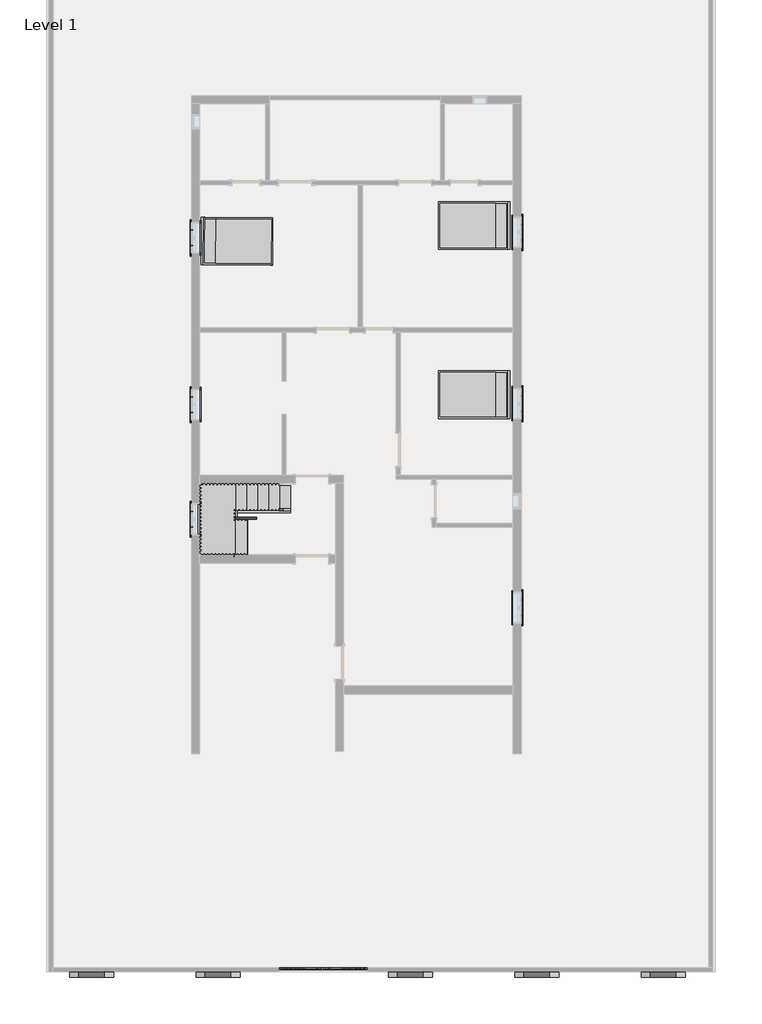
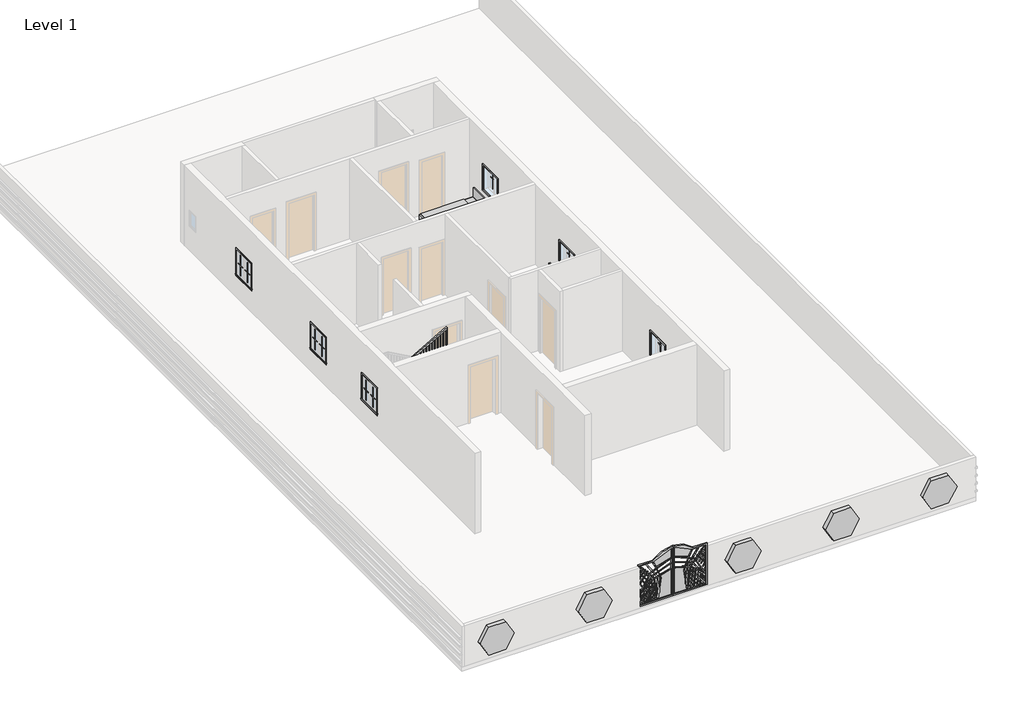
# One storey, part 3 of 3: 26 proxies, 6 members, 3 furniture elements, 1 railing, 1 stair flight.
"""IFC4 building model written with IfcOpenShell, lengths in millimetres."""

from ifc_helpers import new_model, si_unit, frame, origin, place, context, project, spatial, polyline, outline, extrude, faceted_brep, transform, mapped, element, save
from components import generic_models_6bc30956, generic_models_1_generic_models_1_ff25953a, muntin_pattern_2x2_muntin_pattern_2x2_b3fe6957, muntin_pattern_2x2_muntin_pattern_2x2_3e0ecaf2, trim_window_exterior_flat_with_sill_41619996, trim_window_interior_flat_picture_frame_51c85655, bed_17739_bed_17739_15c61121, stair_flight_c1fd4bb9

model = new_model("IFC4")

# Units and contexts
model_context = context("Model", 3, world=origin())
ifc_project = project(units=[si_unit("LENGTHUNIT", "METRE", prefix="MILLI")], contexts=[model_context])

# Site, building, storey
site = spatial("IfcSite", under=ifc_project)
building = spatial("IfcBuilding", under=site)
storey = spatial("IfcBuildingStorey", under=building, Name="Level 1", Elevation=0.0)

# Proxies
placement = place(None, origin())
generic_models_shape = generic_models_6bc30956(model_context)
element("IfcBuildingElementProxy", 1, Name="Generic Models", at=placement, inside=storey, context=model_context, shape_type="MappedRepresentation", body=[
    mapped(generic_models_shape, transform((-2182.3415084, -13739.5284905, 0.0), x_axis=(1.0, 0.0, 0.0), y_axis=(0.0, 1.0, 0.0), z_axis=(0.0, 0.0, 1.0))),
])
generic_models_1_generic_models_1_shape = generic_models_1_generic_models_1_ff25953a(model_context)
element("IfcBuildingElementProxy", 2, Name="Generic Models 1 : Generic Models 1", ObjectType="Generic Models 1 : Generic Models 1", at=placement, inside=storey, context=model_context, shape_type="MappedRepresentation", body=[
    mapped(generic_models_1_generic_models_1_shape, transform((0.0, 0.0, 0.0), x_axis=(1.0, 0.0, 0.0), y_axis=(0.0, 1.0, 0.0), z_axis=(0.0, 0.0, 1.0))),
])
muntin_pattern_2x2_muntin_pattern_2x2_shape = muntin_pattern_2x2_muntin_pattern_2x2_b3fe6957(model_context)
element("IfcBuildingElementProxy", 3, Name="Muntin Pattern_2x2 : Muntin Pattern_2x2", ObjectType="Muntin Pattern_2x2 : Muntin Pattern_2x2", at=placement, inside=storey, context=model_context, shape_type="MappedRepresentation", body=[
    mapped(muntin_pattern_2x2_muntin_pattern_2x2_shape, transform((3307.2334916, 6850.4197267, 984.25), x_axis=(0.0, -1.0, 0.0), y_axis=(1.0, 0.0, 0.0), z_axis=(0.0, 0.0, 1.0))),
])
element("IfcBuildingElementProxy", 4, Name="Muntin Pattern_2x2 : Muntin Pattern_2x2", ObjectType="Muntin Pattern_2x2 : Muntin Pattern_2x2", at=placement, inside=storey, context=model_context, shape_type="MappedRepresentation", body=[
    mapped(muntin_pattern_2x2_muntin_pattern_2x2_shape, transform((3307.2334916, 2106.9697267, 984.25), x_axis=(0.0, -1.0, 0.0), y_axis=(1.0, 0.0, 0.0), z_axis=(0.0, 0.0, 1.0))),
])
element("IfcBuildingElementProxy", 5, Name="Muntin Pattern_2x2 : Muntin Pattern_2x2", ObjectType="Muntin Pattern_2x2 : Muntin Pattern_2x2", at=placement, inside=storey, context=model_context, shape_type="MappedRepresentation", body=[
    mapped(muntin_pattern_2x2_muntin_pattern_2x2_shape, transform((-5817.7165084, 6269.3947267, 984.25), x_axis=(0.0, 1.0, 0.0), y_axis=(-1.0, 0.0, 0.0), z_axis=(0.0, 0.0, 1.0))),
])
element("IfcBuildingElementProxy", 6, Name="Muntin Pattern_2x2 : Muntin Pattern_2x2", ObjectType="Muntin Pattern_2x2 : Muntin Pattern_2x2", at=placement, inside=storey, context=model_context, shape_type="MappedRepresentation", body=[
    mapped(muntin_pattern_2x2_muntin_pattern_2x2_shape, transform((-5817.7165084, 1649.7697267, 984.25), x_axis=(0.0, 1.0, 0.0), y_axis=(-1.0, 0.0, 0.0), z_axis=(0.0, 0.0, 1.0))),
])
element("IfcBuildingElementProxy", 7, Name="Muntin Pattern_2x2 : Muntin Pattern_2x2", ObjectType="Muntin Pattern_2x2 : Muntin Pattern_2x2", at=placement, inside=storey, context=model_context, shape_type="MappedRepresentation", body=[
    mapped(muntin_pattern_2x2_muntin_pattern_2x2_shape, transform((3307.2334916, -3547.7052733, 984.25), x_axis=(0.0, -1.0, 0.0), y_axis=(1.0, 0.0, 0.0), z_axis=(0.0, 0.0, 1.0))),
])
element("IfcBuildingElementProxy", 8, Name="Muntin Pattern_2x2 : Muntin Pattern_2x2", ObjectType="Muntin Pattern_2x2 : Muntin Pattern_2x2", at=placement, inside=storey, context=model_context, shape_type="MappedRepresentation", body=[
    mapped(muntin_pattern_2x2_muntin_pattern_2x2_shape, transform((-5817.7165084, -1522.0552733, 984.25), x_axis=(0.0, 1.0, 0.0), y_axis=(-1.0, 0.0, 0.0), z_axis=(0.0, 0.0, 1.0))),
])
muntin_pattern_2x2_muntin_pattern_2x2_2_shape = muntin_pattern_2x2_muntin_pattern_2x2_3e0ecaf2(model_context)
element("IfcBuildingElementProxy", 9, Name="Muntin Pattern_2x2 : Muntin Pattern_2x2", ObjectType="Muntin Pattern_2x2 : Muntin Pattern_2x2", at=placement, inside=storey, context=model_context, shape_type="MappedRepresentation", body=[
    mapped(muntin_pattern_2x2_muntin_pattern_2x2_2_shape, transform((3307.2334916, 6421.7947267, 984.25), x_axis=(0.0, 1.0, 0.0), y_axis=(-1.0, 0.0, 0.0), z_axis=(0.0, 0.0, 1.0))),
])
element("IfcBuildingElementProxy", 10, Name="Muntin Pattern_2x2 : Muntin Pattern_2x2", ObjectType="Muntin Pattern_2x2 : Muntin Pattern_2x2", at=placement, inside=storey, context=model_context, shape_type="MappedRepresentation", body=[
    mapped(muntin_pattern_2x2_muntin_pattern_2x2_2_shape, transform((3307.2334916, 1678.3447267, 984.25), x_axis=(0.0, 1.0, 0.0), y_axis=(-1.0, 0.0, 0.0), z_axis=(0.0, 0.0, 1.0))),
])
element("IfcBuildingElementProxy", 11, Name="Muntin Pattern_2x2 : Muntin Pattern_2x2", ObjectType="Muntin Pattern_2x2 : Muntin Pattern_2x2", at=placement, inside=storey, context=model_context, shape_type="MappedRepresentation", body=[
    mapped(muntin_pattern_2x2_muntin_pattern_2x2_2_shape, transform((-5817.7165084, 6698.0197267, 984.25), x_axis=(0.0, -1.0, 0.0), y_axis=(1.0, 0.0, 0.0), z_axis=(0.0, 0.0, 1.0))),
])
element("IfcBuildingElementProxy", 12, Name="Muntin Pattern_2x2 : Muntin Pattern_2x2", ObjectType="Muntin Pattern_2x2 : Muntin Pattern_2x2", at=placement, inside=storey, context=model_context, shape_type="MappedRepresentation", body=[
    mapped(muntin_pattern_2x2_muntin_pattern_2x2_2_shape, transform((-5817.7165084, 2078.3947267, 984.25), x_axis=(0.0, -1.0, 0.0), y_axis=(1.0, 0.0, 0.0), z_axis=(0.0, 0.0, 1.0))),
])
element("IfcBuildingElementProxy", 13, Name="Muntin Pattern_2x2 : Muntin Pattern_2x2", ObjectType="Muntin Pattern_2x2 : Muntin Pattern_2x2", at=placement, inside=storey, context=model_context, shape_type="MappedRepresentation", body=[
    mapped(muntin_pattern_2x2_muntin_pattern_2x2_2_shape, transform((3307.2334916, -3976.3302733, 984.25), x_axis=(0.0, 1.0, 0.0), y_axis=(-1.0, 0.0, 0.0), z_axis=(0.0, 0.0, 1.0))),
])
element("IfcBuildingElementProxy", 14, Name="Muntin Pattern_2x2 : Muntin Pattern_2x2", ObjectType="Muntin Pattern_2x2 : Muntin Pattern_2x2", at=placement, inside=storey, context=model_context, shape_type="MappedRepresentation", body=[
    mapped(muntin_pattern_2x2_muntin_pattern_2x2_2_shape, transform((-5817.7165084, -1093.4302733, 984.25), x_axis=(0.0, -1.0, 0.0), y_axis=(1.0, 0.0, 0.0), z_axis=(0.0, 0.0, 1.0))),
])
trim_window_exterior_flat_with_sill_shape = trim_window_exterior_flat_with_sill_41619996(model_context)
element("IfcBuildingElementProxy", 15, Name="Trim-Window-Exterior-Flat : with Sill", ObjectType="Trim-Window-Exterior-Flat : with Sill", at=placement, inside=storey, context=model_context, shape_type="MappedRepresentation", body=[
    mapped(trim_window_exterior_flat_with_sill_shape, transform((3316.7584916, 6636.1072267, 1828.8), x_axis=(0.0, 1.0, 0.0), y_axis=(0.0, 0.0, 1.0), z_axis=(1.0, 0.0, 0.0))),
])
element("IfcBuildingElementProxy", 16, Name="Trim-Window-Exterior-Flat : with Sill", ObjectType="Trim-Window-Exterior-Flat : with Sill", at=placement, inside=storey, context=model_context, shape_type="MappedRepresentation", body=[
    mapped(trim_window_exterior_flat_with_sill_shape, transform((3316.7584916, 1892.6572267, 1828.8), x_axis=(0.0, 1.0, 0.0), y_axis=(0.0, 0.0, 1.0), z_axis=(1.0, 0.0, 0.0))),
])
element("IfcBuildingElementProxy", 17, Name="Trim-Window-Exterior-Flat : with Sill", ObjectType="Trim-Window-Exterior-Flat : with Sill", at=placement, inside=storey, context=model_context, shape_type="MappedRepresentation", body=[
    mapped(trim_window_exterior_flat_with_sill_shape, transform((-5827.2415084, 6483.7072267, 1828.8), x_axis=(0.0, -1.0, 0.0), y_axis=(0.0, 0.0, 1.0), z_axis=(-1.0, 0.0, 0.0))),
])
element("IfcBuildingElementProxy", 18, Name="Trim-Window-Exterior-Flat : with Sill", ObjectType="Trim-Window-Exterior-Flat : with Sill", at=placement, inside=storey, context=model_context, shape_type="MappedRepresentation", body=[
    mapped(trim_window_exterior_flat_with_sill_shape, transform((-5827.2415084, 1864.0822267, 1828.8), x_axis=(0.0, -1.0, 0.0), y_axis=(0.0, 0.0, 1.0), z_axis=(-1.0, 0.0, 0.0))),
])
element("IfcBuildingElementProxy", 19, Name="Trim-Window-Exterior-Flat : with Sill", ObjectType="Trim-Window-Exterior-Flat : with Sill", at=placement, inside=storey, context=model_context, shape_type="MappedRepresentation", body=[
    mapped(trim_window_exterior_flat_with_sill_shape, transform((3316.7584916, -3762.0177733, 1828.8), x_axis=(0.0, 1.0, 0.0), y_axis=(0.0, 0.0, 1.0), z_axis=(1.0, 0.0, 0.0))),
])
element("IfcBuildingElementProxy", 20, Name="Trim-Window-Exterior-Flat : with Sill", ObjectType="Trim-Window-Exterior-Flat : with Sill", at=placement, inside=storey, context=model_context, shape_type="MappedRepresentation", body=[
    mapped(trim_window_exterior_flat_with_sill_shape, transform((-5827.2415084, -1307.7427733, 1828.8), x_axis=(0.0, -1.0, 0.0), y_axis=(0.0, 0.0, 1.0), z_axis=(-1.0, 0.0, 0.0))),
])
trim_window_interior_flat_picture_frame_shape = trim_window_interior_flat_picture_frame_51c85655(model_context)
element("IfcBuildingElementProxy", 21, Name="Trim-Window-Interior-Flat : Picture Frame", ObjectType="Trim-Window-Interior-Flat : Picture Frame", at=placement, inside=storey, context=model_context, shape_type="MappedRepresentation", body=[
    mapped(trim_window_interior_flat_picture_frame_shape, transform((3088.1584916, 6636.1072267, 1828.8), x_axis=(0.0, -1.0, 0.0), y_axis=(0.0, 0.0, 1.0), z_axis=(-1.0, 0.0, 0.0))),
])
element("IfcBuildingElementProxy", 22, Name="Trim-Window-Interior-Flat : Picture Frame", ObjectType="Trim-Window-Interior-Flat : Picture Frame", at=placement, inside=storey, context=model_context, shape_type="MappedRepresentation", body=[
    mapped(trim_window_interior_flat_picture_frame_shape, transform((3088.1584916, 1892.6572267, 1828.8), x_axis=(0.0, -1.0, 0.0), y_axis=(0.0, 0.0, 1.0), z_axis=(-1.0, 0.0, 0.0))),
])
element("IfcBuildingElementProxy", 23, Name="Trim-Window-Interior-Flat : Picture Frame", ObjectType="Trim-Window-Interior-Flat : Picture Frame", at=placement, inside=storey, context=model_context, shape_type="MappedRepresentation", body=[
    mapped(trim_window_interior_flat_picture_frame_shape, transform((-5598.6415084, 6483.7072267, 1828.8), x_axis=(0.0, 1.0, 0.0), y_axis=(0.0, 0.0, 1.0), z_axis=(1.0, 0.0, 0.0))),
])
element("IfcBuildingElementProxy", 24, Name="Trim-Window-Interior-Flat : Picture Frame", ObjectType="Trim-Window-Interior-Flat : Picture Frame", at=placement, inside=storey, context=model_context, shape_type="MappedRepresentation", body=[
    mapped(trim_window_interior_flat_picture_frame_shape, transform((-5598.6415084, 1864.0822267, 1828.8), x_axis=(0.0, 1.0, 0.0), y_axis=(0.0, 0.0, 1.0), z_axis=(1.0, 0.0, 0.0))),
])
element("IfcBuildingElementProxy", 25, Name="Trim-Window-Interior-Flat : Picture Frame", ObjectType="Trim-Window-Interior-Flat : Picture Frame", at=placement, inside=storey, context=model_context, shape_type="MappedRepresentation", body=[
    mapped(trim_window_interior_flat_picture_frame_shape, transform((3088.1584916, -3762.0177733, 1828.8), x_axis=(0.0, -1.0, 0.0), y_axis=(0.0, 0.0, 1.0), z_axis=(-1.0, 0.0, 0.0))),
])
element("IfcBuildingElementProxy", 26, Name="Trim-Window-Interior-Flat : Picture Frame", ObjectType="Trim-Window-Interior-Flat : Picture Frame", at=placement, inside=storey, context=model_context, shape_type="MappedRepresentation", body=[
    mapped(trim_window_interior_flat_picture_frame_shape, transform((-5598.6415084, -1307.7427733, 1828.8), x_axis=(0.0, 1.0, 0.0), y_axis=(0.0, 0.0, 1.0), z_axis=(1.0, 0.0, 0.0))),
])

# Furniture
bed_17739_bed_17739_shape = bed_17739_bed_17739_15c61121(model_context)
element("IfcFurniture", 27, ObjectType="Bed_17739 : Bed_17739", at=placement, inside=storey, context=model_context, shape_type="MappedRepresentation", body=[
    mapped(bed_17739_bed_17739_shape, transform((-4543.6279345, 6394.2844586, 0.0), x_axis=(0.007593038844487308, 0.9999711724650396, 0.0), y_axis=(-0.9999711724650396, 0.007593038844487308, 0.0), z_axis=(0.0, 0.0, 1.0))),
])
element("IfcFurniture", 28, ObjectType="Bed_17739 : Bed_17739", at=placement, inside=storey, context=model_context, shape_type="MappedRepresentation", body=[
    mapped(bed_17739_bed_17739_shape, transform((1983.2584916, 6826.6072267, 0.0), x_axis=(0.0, -1.0, 0.0), y_axis=(1.0, 0.0, 0.0), z_axis=(0.0, 0.0, 1.0))),
])
element("IfcFurniture", 29, ObjectType="Bed_17739 : Bed_17739", at=placement, inside=storey, context=model_context, shape_type="MappedRepresentation", body=[
    mapped(bed_17739_bed_17739_shape, transform((1983.2584916, 2140.3072267, 0.0), x_axis=(0.0, -1.0, 0.0), y_axis=(1.0, 0.0, 0.0), z_axis=(0.0, 0.0, 1.0))),
])

# Members
element("IfcMember", 30, ObjectType="Stringer - 2\" Width", at=placement, inside=storey, context=model_context, shape_type="SweptSolid", body=[
    extrude(outline(polyline([(0.0, -3084.0415084), (207.5983948, -3084.0415084), (1026.0428392, -4557.2415084), (677.3641651, -4557.2415084), (0.0, -3337.9860112), (0.0, -3084.0415084)])), frame((0.0, -1127.4758739, 0.0), z_axis=(0.0, 1.0, 0.0), x_axis=(0.0, 0.0, 1.0)), (0.0, 0.0, 1.0), 50.8),
])
element("IfcMember", 31, ObjectType="Stringer - 2\" Width", at=placement, inside=storey, context=model_context, shape_type="SweptSolid", body=[
    extrude(outline(polyline([(-4608.0415084, -1076.6758739), (-4557.2415084, -1076.6758739), (-4557.2415084, -1256.9427733), (-4608.0415084, -1256.9427733), (-4608.0415084, -1076.6758739)])), frame((0.0, 0.0, 787.4), z_axis=(0.0, 0.0, 1.0), x_axis=(1.0, 0.0, 0.0)), (0.0, 0.0, 1.0), 304.8),
])
element("IfcMember", 32, ObjectType="Stringer - 2\" Width", at=placement, inside=storey, context=model_context, shape_type="SweptSolid", body=[
    extrude(outline(polyline([(1223.5983948, -4608.0415084), (874.9197207, -4608.0415084), (1721.5863873, -3084.0415084), (2070.2650614, -3084.0415084), (1223.5983948, -4608.0415084)])), frame((0.0, -1307.7427733, 0.0), z_axis=(0.0, 1.0, 0.0), x_axis=(0.0, 0.0, 1.0)), (0.0, 0.0, 1.0), 50.8),
])
element("IfcMember", 33, ObjectType="Stringer - 2\" Width", at=placement, inside=storey, context=model_context, shape_type="SweptSolid", body=[
    extrude(outline(polyline([(0.0, -3084.0415084), (207.5983948, -3084.0415084), (1092.2, -4676.3243978), (1092.2, -5303.9460112), (0.0, -3337.9860112), (0.0, -3084.0415084)])), frame((0.0, -317.1427733, 0.0), z_axis=(0.0, 1.0, 0.0), x_axis=(0.0, 0.0, 1.0)), (0.0, 0.0, 1.0), 50.8),
])
element("IfcMember", 34, ObjectType="Stringer - 2\" Width", at=placement, inside=storey, context=model_context, shape_type="SweptSolid", body=[
    extrude(outline(polyline([(-5649.4415084, -266.3427733), (-5598.6415084, -266.3427733), (-5598.6415084, -2298.3427733), (-5649.4415084, -2298.3427733), (-5649.4415084, -266.3427733)])), frame((0.0, 0.0, 787.4), z_axis=(0.0, 0.0, 1.0), x_axis=(1.0, 0.0, 0.0)), (0.0, 0.0, 1.0), 304.8),
])
element("IfcMember", 35, ObjectType="Stringer - 2\" Width", at=placement, inside=storey, context=model_context, shape_type="SweptSolid", body=[
    extrude(outline(polyline([(787.4, -4765.5770056), (1721.5863873, -3084.0415084), (2070.2650614, -3084.0415084), (787.4, -5393.198619), (787.4, -4765.5770056)])), frame((0.0, -2349.1427733, 0.0), z_axis=(0.0, 1.0, 0.0), x_axis=(0.0, 0.0, 1.0)), (0.0, 0.0, 1.0), 50.8),
])

# Railing
element("IfcRailing", 36, ObjectType="Handrail - Rectangular", at=placement, inside=storey, context=model_context, shape_type="SolidModel", body=[
    faceted_brep([(-3084.0415084, -1076.6758739, 1083.7333333), (-3084.0415084, -1076.6758739, 1025.620221), (-3084.0415084, -1025.8758739, 1025.620221), (-3084.0415084, -1025.8758739, 1083.7333333), (-4531.8415084, -1076.6758739, 1888.0666667), (-4582.6415084, -1076.6758739, 1858.1757765), (-4582.6415084, -1025.8758739, 1858.1757765), (-4531.8415084, -1025.8758739, 1888.0666667), (-4531.8415084, -1076.6758739, 1930.4), (-4582.6415084, -1076.6758739, 1879.6), (-4582.6415084, -1025.8758739, 1879.6), (-4531.8415084, -1025.8758739, 1930.4), (-4608.0415084, -1076.6758739, 1930.4), (-4608.0415084, -1076.6758739, 1879.6), (-4658.8415084, -1025.8758739, 1879.6), (-4658.8415084, -1025.8758739, 1930.4), (-4608.0415084, -1152.8758739, 1930.4), (-4608.0415084, -1152.8758739, 1879.6), (-4658.8415084, -1152.8758739, 1879.6), (-4658.8415084, -1152.8758739, 1930.4), (-4608.0415084, -1231.5427733, 1930.4), (-4608.0415084, -1282.3427733, 1879.6), (-4658.8415084, -1282.3427733, 1879.6), (-4658.8415084, -1231.5427733, 1930.4), (-4608.0415084, -1231.5427733, 2142.0666667), (-4608.0415084, -1282.3427733, 2091.2666667), (-4658.8415084, -1282.3427733, 2091.2666667), (-4658.8415084, -1231.5427733, 2142.0666667), (-4608.0415084, -1307.7427733, 2142.0666667), (-4608.0415084, -1307.7427733, 2091.2666667), (-4658.8415084, -1358.5427733, 2091.2666667), (-4658.8415084, -1358.5427733, 2142.0666667), (-4531.8415084, -1307.7427733, 2142.0666667), (-4518.6779062, -1307.7427733, 2091.2666667), (-4518.6779062, -1358.5427733, 2091.2666667), (-4531.8415084, -1358.5427733, 2142.0666667), (-3084.0415084, -1307.7427733, 2946.4), (-3084.0415084, -1358.5427733, 2946.4), (-3084.0415084, -1358.5427733, 2888.2868876), (-3084.0415084, -1307.7427733, 2888.2868876)], [[[0, 1, 2, 3]], [[1, 0, 4, 5]], [[2, 1, 5, 6]], [[3, 2, 6, 7]], [[0, 3, 7, 4]], [[5, 4, 8, 9]], [[6, 5, 9, 10]], [[7, 6, 10, 11]], [[4, 7, 11, 8]], [[9, 8, 12, 13]], [[10, 9, 13, 14]], [[11, 10, 14, 15]], [[8, 11, 15, 12]], [[13, 12, 16, 17]], [[14, 13, 17, 18]], [[15, 14, 18, 19]], [[12, 15, 19, 16]], [[17, 16, 20, 21]], [[18, 17, 21, 22]], [[19, 18, 22, 23]], [[16, 19, 23, 20]], [[21, 20, 24, 25]], [[22, 21, 25, 26]], [[23, 22, 26, 27]], [[20, 23, 27, 24]], [[25, 24, 28, 29]], [[26, 25, 29, 30]], [[27, 26, 30, 31]], [[24, 27, 31, 28]], [[29, 28, 32, 33]], [[30, 29, 33, 34]], [[31, 30, 34, 35]], [[28, 31, 35, 32]], [[36, 37, 38, 39]], [[33, 32, 36, 39]], [[34, 33, 39, 38]], [[35, 34, 38, 37]], [[32, 35, 37, 36]]]),
    extrude(outline(polyline([(2868.8841099, -3118.9665084), (1862.6666667, -3118.9665084), (1862.6666667, -3099.9165084), (2879.4674432, -3099.9165084), (2868.8841099, -3118.9665084)])), frame((0.0, -1342.6677733, 0.0), z_axis=(0.0, 1.0, 0.0), x_axis=(0.0, 0.0, 1.0)), (0.0, 0.0, 1.0), 19.05),
    extrude(outline(polyline([(2812.4396654, -3220.5665084), (1862.6666667, -3220.5665084), (1862.6666667, -3201.5165084), (2823.0229988, -3201.5165084), (2812.4396654, -3220.5665084)])), frame((0.0, -1342.6677733, 0.0), z_axis=(0.0, 1.0, 0.0), x_axis=(0.0, 0.0, 1.0)), (0.0, 0.0, 1.0), 19.05),
    extrude(outline(polyline([(2755.995221, -3322.1665084), (1862.6666667, -3322.1665084), (1862.6666667, -3303.1165084), (2766.5785543, -3303.1165084), (2755.995221, -3322.1665084)])), frame((0.0, -1342.6677733, 0.0), z_axis=(0.0, 1.0, 0.0), x_axis=(0.0, 0.0, 1.0)), (0.0, 0.0, 1.0), 19.05),
    extrude(outline(polyline([(2699.5507765, -3423.7665084), (1693.3333333, -3423.7665084), (1693.3333333, -3404.7165084), (2710.1341099, -3404.7165084), (2699.5507765, -3423.7665084)])), frame((0.0, -1342.6677733, 0.0), z_axis=(0.0, 1.0, 0.0), x_axis=(0.0, 0.0, 1.0)), (0.0, 0.0, 1.0), 19.05),
    extrude(outline(polyline([(2643.1063321, -3525.3665084), (1693.3333333, -3525.3665084), (1693.3333333, -3506.3165084), (2653.6896654, -3506.3165084), (2643.1063321, -3525.3665084)])), frame((0.0, -1342.6677733, 0.0), z_axis=(0.0, 1.0, 0.0), x_axis=(0.0, 0.0, 1.0)), (0.0, 0.0, 1.0), 19.05),
    extrude(outline(polyline([(2586.6618876, -3626.9665084), (1693.3333333, -3626.9665084), (1693.3333333, -3607.9165084), (2597.245221, -3607.9165084), (2586.6618876, -3626.9665084)])), frame((0.0, -1342.6677733, 0.0), z_axis=(0.0, 1.0, 0.0), x_axis=(0.0, 0.0, 1.0)), (0.0, 0.0, 1.0), 19.05),
    extrude(outline(polyline([(2530.2174432, -3728.5665084), (1524.0, -3728.5665084), (1524.0, -3709.5165084), (2540.8007765, -3709.5165084), (2530.2174432, -3728.5665084)])), frame((0.0, -1342.6677733, 0.0), z_axis=(0.0, 1.0, 0.0), x_axis=(0.0, 0.0, 1.0)), (0.0, 0.0, 1.0), 19.05),
    extrude(outline(polyline([(2473.7729988, -3830.1665084), (1524.0, -3830.1665084), (1524.0, -3811.1165084), (2484.3563321, -3811.1165084), (2473.7729988, -3830.1665084)])), frame((0.0, -1342.6677733, 0.0), z_axis=(0.0, 1.0, 0.0), x_axis=(0.0, 0.0, 1.0)), (0.0, 0.0, 1.0), 19.05),
    extrude(outline(polyline([(2417.3285543, -3931.7665084), (1524.0, -3931.7665084), (1524.0, -3912.7165084), (2427.9118876, -3912.7165084), (2417.3285543, -3931.7665084)])), frame((0.0, -1342.6677733, 0.0), z_axis=(0.0, 1.0, 0.0), x_axis=(0.0, 0.0, 1.0)), (0.0, 0.0, 1.0), 19.05),
    extrude(outline(polyline([(2360.8841099, -4033.3665084), (1354.6666667, -4033.3665084), (1354.6666667, -4014.3165084), (2371.4674432, -4014.3165084), (2360.8841099, -4033.3665084)])), frame((0.0, -1342.6677733, 0.0), z_axis=(0.0, 1.0, 0.0), x_axis=(0.0, 0.0, 1.0)), (0.0, 0.0, 1.0), 19.05),
    extrude(outline(polyline([(2304.4396654, -4134.9665084), (1354.6666667, -4134.9665084), (1354.6666667, -4115.9165084), (2315.0229988, -4115.9165084), (2304.4396654, -4134.9665084)])), frame((0.0, -1342.6677733, 0.0), z_axis=(0.0, 1.0, 0.0), x_axis=(0.0, 0.0, 1.0)), (0.0, 0.0, 1.0), 19.05),
    extrude(outline(polyline([(2247.995221, -4236.5665084), (1354.6666667, -4236.5665084), (1354.6666667, -4217.5165084), (2258.5785543, -4217.5165084), (2247.995221, -4236.5665084)])), frame((0.0, -1342.6677733, 0.0), z_axis=(0.0, 1.0, 0.0), x_axis=(0.0, 0.0, 1.0)), (0.0, 0.0, 1.0), 19.05),
    extrude(outline(polyline([(2191.5507765, -4338.1665084), (1185.3333333, -4338.1665084), (1185.3333333, -4319.1165084), (2202.1341099, -4319.1165084), (2191.5507765, -4338.1665084)])), frame((0.0, -1342.6677733, 0.0), z_axis=(0.0, 1.0, 0.0), x_axis=(0.0, 0.0, 1.0)), (0.0, 0.0, 1.0), 19.05),
    extrude(outline(polyline([(2135.1063321, -4439.7665084), (1185.3333333, -4439.7665084), (1185.3333333, -4420.7165084), (2145.6896654, -4420.7165084), (2135.1063321, -4439.7665084)])), frame((0.0, -1342.6677733, 0.0), z_axis=(0.0, 1.0, 0.0), x_axis=(0.0, 0.0, 1.0)), (0.0, 0.0, 1.0), 19.05),
    extrude(outline(polyline([(2078.6618876, -4541.3665084), (1185.3333333, -4541.3665084), (1185.3333333, -4522.3165084), (2089.245221, -4522.3165084), (2078.6618876, -4541.3665084)])), frame((0.0, -1342.6677733, 0.0), z_axis=(0.0, 1.0, 0.0), x_axis=(0.0, 0.0, 1.0)), (0.0, 0.0, 1.0), 19.05),
    extrude(outline(polyline([(-4623.9165084, -1244.9508739), (-4623.9165084, -1264.0008739), (-4642.9665084, -1264.0008739), (-4642.9665084, -1244.9508739), (-4623.9165084, -1244.9508739)])), frame((0.0, 0.0, 1016.0), z_axis=(0.0, 0.0, 1.0), x_axis=(1.0, 0.0, 0.0)), (0.0, 0.0, 1.0), 1075.2666667),
    extrude(outline(polyline([(-4623.9165084, -1143.3508739), (-4623.9165084, -1162.4008739), (-4642.9665084, -1162.4008739), (-4642.9665084, -1143.3508739), (-4623.9165084, -1143.3508739)])), frame((0.0, 0.0, 1016.0), z_axis=(0.0, 0.0, 1.0), x_axis=(1.0, 0.0, 0.0)), (0.0, 0.0, 1.0), 863.6),
    extrude(outline(polyline([(-4598.5165084, -1060.8008739), (-4617.5665084, -1060.8008739), (-4617.5665084, -1041.7508739), (-4598.5165084, -1041.7508739), (-4598.5165084, -1060.8008739)])), frame((0.0, 0.0, 1016.0), z_axis=(0.0, 0.0, 1.0), x_axis=(1.0, 0.0, 0.0)), (0.0, 0.0, 1.0), 863.6),
    extrude(outline(polyline([(1821.1341099, -4515.9665084), (846.6666667, -4515.9665084), (846.6666667, -4496.9165084), (1810.5507765, -4496.9165084), (1821.1341099, -4515.9665084)])), frame((0.0, -1060.8008739, 0.0), z_axis=(0.0, 1.0, 0.0), x_axis=(0.0, 0.0, 1.0)), (0.0, 0.0, 1.0), 19.05),
    extrude(outline(polyline([(1764.6896654, -4414.3665084), (846.6666667, -4414.3665084), (846.6666667, -4395.3165084), (1754.1063321, -4395.3165084), (1764.6896654, -4414.3665084)])), frame((0.0, -1060.8008739, 0.0), z_axis=(0.0, 1.0, 0.0), x_axis=(0.0, 0.0, 1.0)), (0.0, 0.0, 1.0), 19.05),
    extrude(outline(polyline([(1708.245221, -4312.7665084), (846.6666667, -4312.7665084), (846.6666667, -4293.7165084), (1697.6618876, -4293.7165084), (1708.245221, -4312.7665084)])), frame((0.0, -1060.8008739, 0.0), z_axis=(0.0, 1.0, 0.0), x_axis=(0.0, 0.0, 1.0)), (0.0, 0.0, 1.0), 19.05),
    extrude(outline(polyline([(1651.8007765, -4211.1665084), (677.3333333, -4211.1665084), (677.3333333, -4192.1165084), (1641.2174432, -4192.1165084), (1651.8007765, -4211.1665084)])), frame((0.0, -1060.8008739, 0.0), z_axis=(0.0, 1.0, 0.0), x_axis=(0.0, 0.0, 1.0)), (0.0, 0.0, 1.0), 19.05),
    extrude(outline(polyline([(1595.3563321, -4109.5665084), (677.3333333, -4109.5665084), (677.3333333, -4090.5165084), (1584.7729988, -4090.5165084), (1595.3563321, -4109.5665084)])), frame((0.0, -1060.8008739, 0.0), z_axis=(0.0, 1.0, 0.0), x_axis=(0.0, 0.0, 1.0)), (0.0, 0.0, 1.0), 19.05),
    extrude(outline(polyline([(1538.9118876, -4007.9665084), (677.3333333, -4007.9665084), (677.3333333, -3988.9165084), (1528.3285543, -3988.9165084), (1538.9118876, -4007.9665084)])), frame((0.0, -1060.8008739, 0.0), z_axis=(0.0, 1.0, 0.0), x_axis=(0.0, 0.0, 1.0)), (0.0, 0.0, 1.0), 19.05),
    extrude(outline(polyline([(1482.4674432, -3906.3665084), (508.0, -3906.3665084), (508.0, -3887.3165084), (1471.8841099, -3887.3165084), (1482.4674432, -3906.3665084)])), frame((0.0, -1060.8008739, 0.0), z_axis=(0.0, 1.0, 0.0), x_axis=(0.0, 0.0, 1.0)), (0.0, 0.0, 1.0), 19.05),
    extrude(outline(polyline([(1426.0229988, -3804.7665084), (508.0, -3804.7665084), (508.0, -3785.7165084), (1415.4396654, -3785.7165084), (1426.0229988, -3804.7665084)])), frame((0.0, -1060.8008739, 0.0), z_axis=(0.0, 1.0, 0.0), x_axis=(0.0, 0.0, 1.0)), (0.0, 0.0, 1.0), 19.05),
    extrude(outline(polyline([(1369.5785543, -3703.1665084), (508.0, -3703.1665084), (508.0, -3684.1165084), (1358.995221, -3684.1165084), (1369.5785543, -3703.1665084)])), frame((0.0, -1060.8008739, 0.0), z_axis=(0.0, 1.0, 0.0), x_axis=(0.0, 0.0, 1.0)), (0.0, 0.0, 1.0), 19.05),
    extrude(outline(polyline([(1313.1341099, -3601.5665084), (338.6666667, -3601.5665084), (338.6666667, -3582.5165084), (1302.5507765, -3582.5165084), (1313.1341099, -3601.5665084)])), frame((0.0, -1060.8008739, 0.0), z_axis=(0.0, 1.0, 0.0), x_axis=(0.0, 0.0, 1.0)), (0.0, 0.0, 1.0), 19.05),
    extrude(outline(polyline([(1256.6896654, -3499.9665084), (338.6666667, -3499.9665084), (338.6666667, -3480.9165084), (1246.1063321, -3480.9165084), (1256.6896654, -3499.9665084)])), frame((0.0, -1060.8008739, 0.0), z_axis=(0.0, 1.0, 0.0), x_axis=(0.0, 0.0, 1.0)), (0.0, 0.0, 1.0), 19.05),
    extrude(outline(polyline([(1200.245221, -3398.3665084), (338.6666667, -3398.3665084), (338.6666667, -3379.3165084), (1189.6618876, -3379.3165084), (1200.245221, -3398.3665084)])), frame((0.0, -1060.8008739, 0.0), z_axis=(0.0, 1.0, 0.0), x_axis=(0.0, 0.0, 1.0)), (0.0, 0.0, 1.0), 19.05),
    extrude(outline(polyline([(1143.8007765, -3296.7665084), (169.3333333, -3296.7665084), (169.3333333, -3277.7165084), (1133.2174432, -3277.7165084), (1143.8007765, -3296.7665084)])), frame((0.0, -1060.8008739, 0.0), z_axis=(0.0, 1.0, 0.0), x_axis=(0.0, 0.0, 1.0)), (0.0, 0.0, 1.0), 19.05),
    extrude(outline(polyline([(1087.3563321, -3195.1665084), (169.3333333, -3195.1665084), (169.3333333, -3176.1165084), (1076.7729988, -3176.1165084), (1087.3563321, -3195.1665084)])), frame((0.0, -1060.8008739, 0.0), z_axis=(0.0, 1.0, 0.0), x_axis=(0.0, 0.0, 1.0)), (0.0, 0.0, 1.0), 19.05),
    extrude(outline(polyline([(-4623.9165084, -1323.6177733), (-4623.9165084, -1342.6677733), (-4642.9665084, -1342.6677733), (-4642.9665084, -1323.6177733), (-4623.9165084, -1323.6177733)])), frame((0.0, 0.0, 1016.0), z_axis=(0.0, 0.0, 1.0), x_axis=(1.0, 0.0, 0.0)), (0.0, 0.0, 1.0), 1075.2666667),
    extrude(outline(polyline([(-4623.9165084, -1060.8008739), (-4642.9665084, -1060.8008739), (-4642.9665084, -1041.7508739), (-4623.9165084, -1041.7508739), (-4623.9165084, -1060.8008739)])), frame((0.0, 0.0, 1016.0), z_axis=(0.0, 0.0, 1.0), x_axis=(1.0, 0.0, 0.0)), (0.0, 0.0, 1.0), 863.6),
    extrude(outline(polyline([(2877.7035543, -3103.0915084), (1862.6666667, -3103.0915084), (1862.6666667, -3084.0415084), (2888.2868876, -3084.0415084), (2877.7035543, -3103.0915084)])), frame((0.0, -1342.6677733, 0.0), z_axis=(0.0, 1.0, 0.0), x_axis=(0.0, 0.0, 1.0)), (0.0, 0.0, 1.0), 19.05),
    extrude(outline(polyline([(1036.2035543, -3103.0915084), (169.3333333, -3103.0915084), (169.3333333, -3084.0415084), (1025.620221, -3084.0415084), (1036.2035543, -3103.0915084)])), frame((0.0, -1060.8008739, 0.0), z_axis=(0.0, 1.0, 0.0), x_axis=(0.0, 0.0, 1.0)), (0.0, 0.0, 1.0), 19.05),
])

# Stair flight
stair_flight_shape = stair_flight_c1fd4bb9(model_context)
element("IfcStairFlight", 37, ObjectType="2\" Tread 1\" Nosing 1/4\" Riser", at=placement, inside=storey, context=model_context, shape_type="MappedRepresentation", body=[
    mapped(stair_flight_shape, transform((0.0, 0.0, 0.0), x_axis=(1.0, 0.0, 0.0), y_axis=(0.0, 1.0, 0.0), z_axis=(0.0, 0.0, 1.0))),
])

save(model, "model.ifc")

# Revit data of these elements
# Type
#   m.s. sheet = none
#   2" x2" pipe = none
#   1"x1"pipe = none
#   Default Elevation = 0
# Type "Muntin Pattern_2x2 : Muntin Pattern_2x2"
#   Width [instance default] = 4' - 0"
#   Thickness = 0' - 0 1/2"
#   Height [instance default] = 4' - 0"
#   Distance = 0' - 0 3/4"
#   Interior Material [instance default] = none
#   Exterior Material [instance default] = none
#   Default Elevation = 0
# Type "Trim-Window-Exterior-Flat : with Sill"
#   Trim Width = 0' - 2 1/4"
#   Trim Thickness_Picture Frame = 0' - 1 1/4"
#   Trim Thickness_with Sill = 0' - 0 3/4"
#   Sill Thickness = 0' - 1 1/4"
#   Opening Width [instance default] = 2' - 0"
#   Opening Height [instance default] = 3' - 0"
#   Default Elevation = 4' - 0"
#   Sill = yes
#   Picture Frame = no
#   Trim Material [instance default] = none
# Type "Trim-Window-Interior-Flat : Picture Frame"
#   Trim Thickness_Picture Frame = 0' - 1 1/4"
#   Trim Width = 0' - 2 1/4"
#   Trim Thickness_with Sill = 0' - 0 3/4"
#   Sill Thickness = 0' - 1 1/4"
#   Opening Width [instance default] = 2' - 0"
#   Opening Height [instance default] = 3' - 0"
#   Default Elevation = 4' - 0"
#   Sill = no
#   Picture Frame = yes
#   Trim Material [instance default] = none
# Type "Bed_17739 : Bed_17739"
#   Default Elevation = 0
# Type "Handrail - Rectangular"
#   Assembly Code = "C2010400"
#   built-in parameter 1008612 = 0.0416667 (stored number, unit not read)
#   built-in parameter 1008611 = 0.0416667 (stored number, unit not read)
#   built-in parameter 1008609 = 0.333333 (stored number, unit not read)
#   built-in parameter 1008604 = 0.166667 (stored number, unit not read)
#   built-in parameter 1008603 = 0.166667 (stored number, unit not read)
#   Railing Height = 3' - 0"
#   built-in parameter 1008630 = 2
#   built-in parameter 1008610 = 2
#   built-in parameter 1008618 = Baluster - Square : 3/4"
# Element 1 (IfcBuildingElementProxy)
#   Phase Created = New Construction
#   Materials on its faces: "r1"
# Element 2 (IfcBuildingElementProxy, "Generic Models 1 : Generic Models 1")
#   Phase Created = New Construction
#   Materials on its faces: "Brick, Common"
# Elements 3, 4, 5, 6, 7, 8, 9, 10, 11, 12, 13, 14 (IfcBuildingElementProxy, "Muntin Pattern_2x2 : Muntin Pattern_2x2")
#   Width = 0' - 11 5/8"
#   Height = 2' - 6 1/2"
#   Interior Material = Wood - Stained
#   Exterior Material = Clad - White
#   Phase Created = New Construction
#   Materials on its faces: "Clad - White", "Wood - Stained"
# Elements 15, 16, 17, 18, 19, 20 (IfcBuildingElementProxy, "Trim-Window-Exterior-Flat : with Sill")
#   Opening Width = 2' - 10"
#   Opening Height = 3' - 0"
#   Trim Material = Clad - White
#   Phase Created = New Construction
#   Materials on its faces: "Clad - White"
# Elements 21, 22, 23, 24, 25, 26 (IfcBuildingElementProxy, "Trim-Window-Interior-Flat : Picture Frame")
#   Opening Width = 2' - 10"
#   Opening Height = 3' - 0"
#   Trim Material = Wood - Stained
#   Phase Created = New Construction
#   Materials on its faces: "Wood - Stained"
# Elements 27, 28, 29 (IfcFurniture, "Bed_17739 : Bed_17739")
#   Phase Created = New Construction
#   Materials on its faces: "legs", "sheets", "bed frame", "Blanket"
# Elements 30, 31, 32, 33, 34, 35 (IfcMember, "Stringer - 2\" Width")
#   Phase Created = New Construction
# Element 36 (IfcRailing, "Handrail - Rectangular")
#   Phase Created = New Construction
# Element 37 (IfcStairFlight, "2\" Tread 1\" Nosing 1/4\" Riser")
#   Phase Created = New Construction
# Materials
#   "r1": class "Generic", colour RGB 120 120 120, transparency 0, Cost = 0
#   "Brick, Common": class "Masonry", colour RGB 170 98 104, transparency 0, Description = "Common brick", Cost = 0
#   "Clad - White": class "Wood", colour RGB 242 242 238, transparency 0, Cost = 0
#   "Wood - Stained": class "Wood", colour RGB 224 178 126, transparency 0, Cost = 0
#   "legs": colour RGB 90 73 37, transparency 0, Cost = 0
#   "sheets": colour RGB 200 195 176, transparency 0, Cost = 0
#   "bed frame": colour RGB 90 73 37, transparency 0, Cost = 0
#   "Blanket": class "System", colour RGB 59 0 1, transparency 0, Cost = 0
